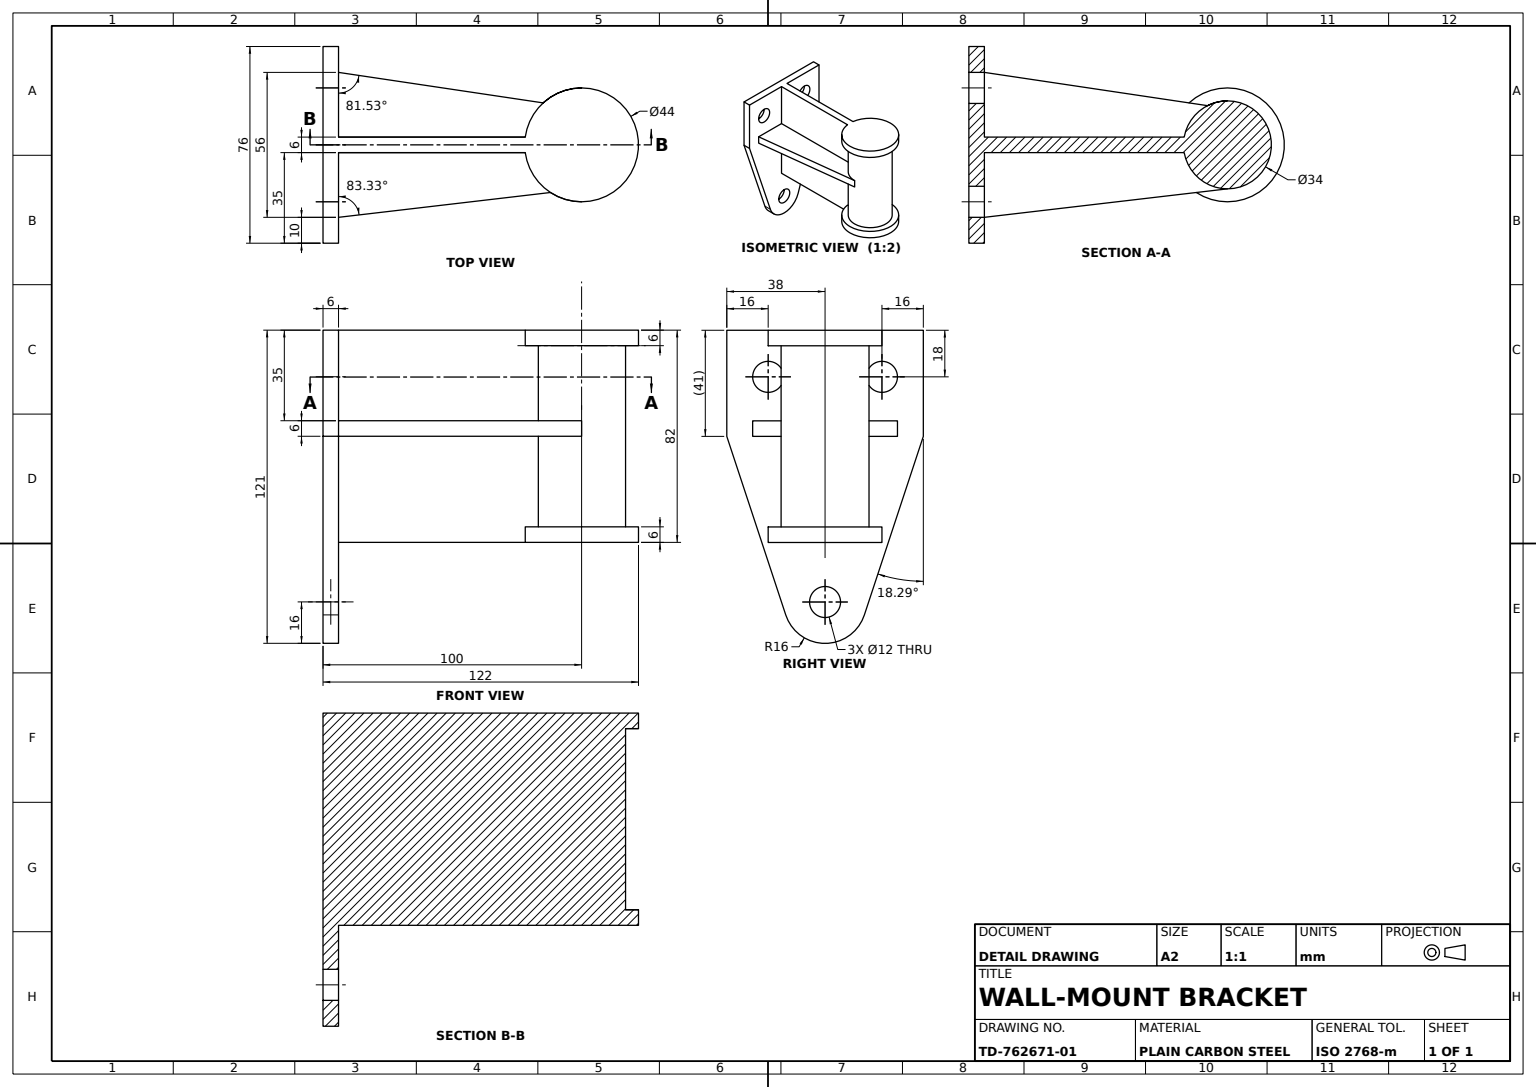
from build123d import *

# Parameters (mm, degrees)
POST_34_DEPTH              = 82
SKETCH1_4_R                = 22
SKETCH1_4_R_2              = 17
BASE_COLLAR_44_DEPTH       = 6
TOP_START                  = -6
TOP_CAP_SKETCH_R           = 22
TOP_CAP_SKETCH_R_2         = 17
TOP_CAP_DEPTH              = 6
SUPPORT_ARM_PROFILE_W      = 94
SUPPORT_ARM_PROFILE_H      = 3
SUPPORT_ARM_PROFILE_W_2    = 6
SUPPORT_ARM_PROFILE_H_2    = 35
SUPPORT_ARM_DEPTH          = 41
WALL_START                 = -6
WALL_PLATE_DEPTH           = 6
LOWER_PLATE_LOBE_SKETCH_R  = 6
LOWER_PLATE_LOBE_DEPTH     = 6
MOUNTING_HOLES_SKETCH_R    = 6
MOUNTING_HOLES_2X_12_DEPTH = 6
STIFFENER_RIB_SKETCH_W     = 94
STIFFENER_RIB_SKETCH_H     = 6
STIFFENER_RIB_DEPTH        = 41


with BuildPart() as part:
    # Post and Collar Profile → Post _34 (new body)
    with BuildSketch(Plane(origin=(0, 0, 0), x_dir=(1, 0, 0), z_dir=(0, 1, 0))):
        with BuildLine():
            ThreePointArc((17, 0), (0, 17), (-17, 0))
            Line((-17, 0), (17, 0))
        make_face()
        with BuildLine():
            Line((17, 0), (-17, 0))
            ThreePointArc((-17, 0), (0, -17), (17, 0))
        make_face()
        with BuildLine():
            ThreePointArc((17, 0), (0, 17), (-17, 0))
            Line((-17, 0), (17, 0))
        make_face()
        with BuildLine():
            Line((17, 0), (-17, 0))
            ThreePointArc((-17, 0), (0, -17), (17, 0))
        make_face()
    extrude(amount=POST_34_DEPTH)

    # Sketch1_4 → Base Collar _44 (add)
    with BuildSketch(Plane(origin=(0, 0, 0), x_dir=(1, 0, 0), z_dir=(0, 1, 0))):
        with Locations(Location((0, 0, 0), (0, 0, 270))):
            Circle(SKETCH1_4_R)
        with Locations(Location((0, 0, 0), (0, 0, 270))):
            Circle(SKETCH1_4_R_2, mode=Mode.SUBTRACT)
    extrude(amount=BASE_COLLAR_44_DEPTH)

    # Top Cap Sketch → Top Cap (add)
    with BuildSketch(Plane(origin=(0, 82, 0), x_dir=(1, 0, 0), z_dir=(0, 1, 0)).offset(TOP_START)):
        with Locations(Location((0, 0, 0), (0, 0, 270))):
            Circle(TOP_CAP_SKETCH_R)
        with Locations(Location((0, 0, 0), (0, 0, 270))):
            Circle(TOP_CAP_SKETCH_R_2, mode=Mode.SUBTRACT)
    extrude(amount=TOP_CAP_DEPTH)

    # Support Arm Profile → Support Arm (add)
    with BuildSketch(Plane(origin=(0, 82, 0), x_dir=(1, 0, 0), z_dir=(0, 1, 0))):
        with Locations((-47, -1.5)):
            Rectangle(SUPPORT_ARM_PROFILE_W, SUPPORT_ARM_PROFILE_H)
        with Locations((-47, 1.5)):
            Rectangle(SUPPORT_ARM_PROFILE_W, SUPPORT_ARM_PROFILE_H)
        with Locations((-97, -20.5)):
            Rectangle(SUPPORT_ARM_PROFILE_W_2, SUPPORT_ARM_PROFILE_H_2)
        with Locations((-97, -1.5)):
            Rectangle(SUPPORT_ARM_PROFILE_W_2, SUPPORT_ARM_PROFILE_H)
        with Locations((-97, 1.5)):
            Rectangle(SUPPORT_ARM_PROFILE_W_2, SUPPORT_ARM_PROFILE_H)
        with Locations((-97, 20.5)):
            Rectangle(SUPPORT_ARM_PROFILE_W_2, SUPPORT_ARM_PROFILE_H_2)
    extrude(amount=-SUPPORT_ARM_DEPTH)

    # Wall Plate Sketch → Wall Plate (add)
    with BuildSketch(Plane(origin=(0, 47, 0), x_dir=(1, 0, 0), z_dir=(0, 1, 0)).offset(WALL_START)):
        with BuildLine():
            Line((-16.733200531, -3), (-94, -3))
            Line((-94, -3), (-94, -28))
            Line((-94, -28), (0, -17))
            ThreePointArc((0, -17), (-10.908712115, -13.03840481), (-16.733200531, -3))
        make_face()
        with BuildLine():
            Line((-94, 3), (-16.733200531, 3))
            ThreePointArc((-16.733200531, 3), (-13.649862572, 10.133175798), (-7.714262086, 15.148932651))
            Line((-7.714262086, 15.148932651), (-94, 28))
            Line((-94, 28), (-94, 3))
        make_face()
    extrude(amount=WALL_PLATE_DEPTH)

    # Lower Plate Lobe Sketch → Lower Plate Lobe (add)
    with BuildSketch(Plane.ZY.offset(100)):
        with BuildLine():
            Line((38, 41), (-38, 41))
            Line((-38, 41), (-15.192006216, -28.020253691))
            ThreePointArc((-15.192006216, -28.020253691), (0, -39), (15.192006216, -28.020253691))
            Line((15.192006216, -28.020253691), (16.850967302, -23))
            Line((16.850967302, -23), (38, 41))
        make_face()
        with Locations((0, -23)):
            Circle(LOWER_PLATE_LOBE_SKETCH_R, mode=Mode.SUBTRACT)
    extrude(amount=-LOWER_PLATE_LOBE_DEPTH)

    # Mounting Holes Sketch → Mounting Holes 2x_12 (cut)
    with BuildSketch(Plane.ZY.offset(100)):
        with Locations((-22, 64)):
            Circle(MOUNTING_HOLES_SKETCH_R)
        with Locations((22, 64)):
            Circle(MOUNTING_HOLES_SKETCH_R)
    extrude(amount=-MOUNTING_HOLES_2X_12_DEPTH, mode=Mode.SUBTRACT)

    # Stiffener Rib Sketch → Stiffener Rib (add)
    with BuildSketch(Plane.XZ):
        with Locations((-47, 0)):
            Rectangle(STIFFENER_RIB_SKETCH_W, STIFFENER_RIB_SKETCH_H)
    extrude(amount=-STIFFENER_RIB_DEPTH)


solid = part.part
